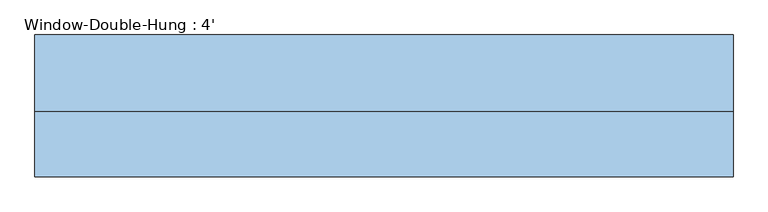
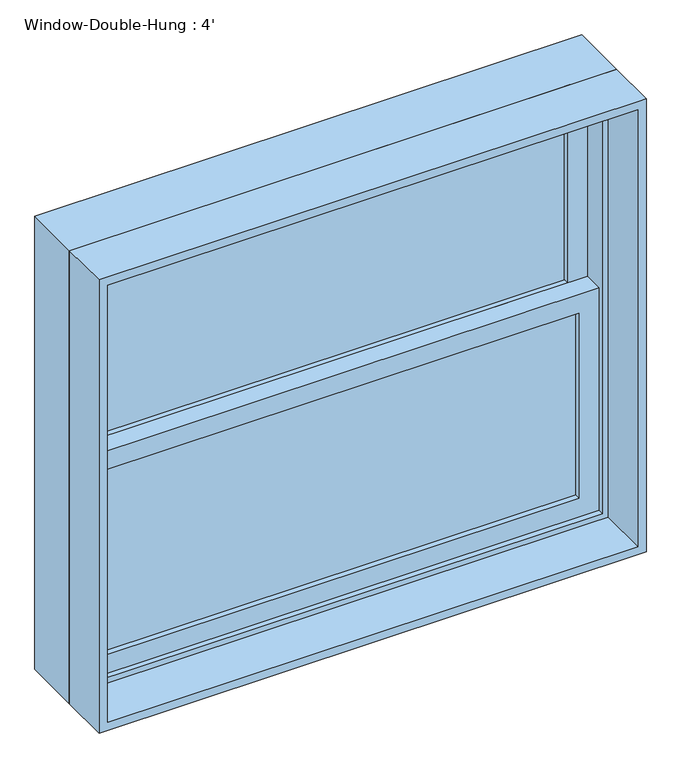
"""IFC4 building model written with IfcOpenShell, lengths in millimetres: window geometry, Window-Double-Hung : 4'."""

from ifc_helpers import new_model, si_unit, frame, origin, place, context, project, spatial, polyline, outline, extrude, source, transform, mapped, element, save


def window_double_hung_4_eadb0177(model_context):
    return source(origin(), model_context, "Body", "SweptSolid", [
        extrude(outline(polyline([(533.4, 44.45), (533.4, 38.1), (-533.4, 38.1), (-533.4, 44.45), (533.4, 44.45)])), frame((0.0, 0.0, 990.6), z_axis=(0.0, 0.0, 1.0), x_axis=(1.0, 0.0, 0.0)), (0.0, 0.0, 1.0), 434.975),
        extrude(outline(polyline([(-533.4, 31.75), (533.4, 31.75), (533.4, 25.4), (-533.4, 25.4), (-533.4, 31.75)])), frame((0.0, 0.0, 990.6), z_axis=(0.0, 0.0, 1.0), x_axis=(1.0, 0.0, 0.0)), (0.0, 0.0, 1.0), 434.975),
        extrude(outline(polyline([(533.4, 88.9), (533.4, 82.55), (-533.4, 82.55), (-533.4, 88.9), (533.4, 88.9)])), frame((0.0, 0.0, 1470.025), z_axis=(0.0, 0.0, 1.0), x_axis=(1.0, 0.0, 0.0)), (0.0, 0.0, 1.0), 434.975),
        extrude(outline(polyline([(-533.4, 76.2), (533.4, 76.2), (533.4, 69.85), (-533.4, 69.85), (-533.4, 76.2)])), frame((0.0, 0.0, 1470.025), z_axis=(0.0, 0.0, 1.0), x_axis=(1.0, 0.0, 0.0)), (0.0, 0.0, 1.0), 434.975),
        extrude(outline(polyline([(1470.025, -577.85), (946.15, -577.85), (946.15, 577.85), (1470.025, 577.85), (1470.025, -577.85)]), holes=[polyline([(1425.575, 533.4), (990.6, 533.4), (990.6, -533.4), (1425.575, -533.4), (1425.575, 533.4)])]), frame((0.0, 12.7, 0.0), z_axis=(0.0, 1.0, 0.0), x_axis=(0.0, 0.0, 1.0)), (0.0, 0.0, 1.0), 44.45),
        extrude(outline(polyline([(1949.45, -577.85), (1425.575, -577.85), (1425.575, 577.85), (1949.45, 577.85), (1949.45, -577.85)]), holes=[polyline([(1905.0, 533.4), (1470.025, 533.4), (1470.025, -533.4), (1905.0, -533.4), (1905.0, 533.4)])]), frame((0.0, 57.15, 0.0), z_axis=(0.0, 1.0, 0.0), x_axis=(0.0, 0.0, 1.0)), (0.0, 0.0, 1.0), 44.45),
        extrude(outline(polyline([(1981.2, -609.6), (914.4, -609.6), (914.4, 609.6), (1981.2, 609.6), (1981.2, -609.6)]), holes=[polyline([(1949.45, 577.85), (946.15, 577.85), (946.15, -577.85), (1949.45, -577.85), (1949.45, 577.85)])]), frame((0.0, 0.0, 0.0), z_axis=(0.0, 1.0, 0.0), x_axis=(0.0, 0.0, 1.0)), (0.0, 0.0, 1.0), 133.35),
        extrude(outline(polyline([(1981.2, 609.6), (1981.2, -609.6), (914.4, -609.6), (914.4, 609.6), (1981.2, 609.6)]), holes=[polyline([(1962.15, 590.55), (933.45, 590.55), (933.45, -590.55), (1962.15, -590.55), (1962.15, 590.55)])]), frame((0.0, -114.3, 0.0), z_axis=(0.0, 1.0, 0.0), x_axis=(0.0, 0.0, 1.0)), (0.0, 0.0, 1.0), 114.3),
    ])


if __name__ == "__main__":
    model = new_model("IFC4")
    model_context = context("Model", 3, world=origin())
    ifc_project = project(units=[si_unit("LENGTHUNIT", "METRE", prefix="MILLI")], contexts=[model_context])
    site = spatial("IfcSite", under=ifc_project)
    building = spatial("IfcBuilding", under=site)
    placement = place(None, origin())
    window_double_hung_4_shape = window_double_hung_4_eadb0177(model_context)
    element("IfcWindow", 1, ObjectType="Window-Double-Hung : 4'", at=placement, inside=building, context=model_context, shape_type="MappedRepresentation", body=[
        mapped(window_double_hung_4_shape, transform((0.0, 0.0, 0.0), x_axis=(1.0, 0.0, 0.0), y_axis=(0.0, 1.0, 0.0), z_axis=(0.0, 0.0, 1.0))),
    ])
    save(model, "model.ifc")

# Revit data of these elements
# Type "Window-Double-Hung : 4'"
#   Type Mark = "18"
#   Fire Rating = "0.5h"
#   Construction Type Id = "DG-DR"
#   Assembly Code = "B2020100"
#   Analytic Construction = "Double glazing - domestic"
#   Wall Thickness [instance default] = 0' - 6"
#   Window Inset [instance default] = 0' - 0"
#   Visual Light Transmittance = 0.81
#   Thermal Resistance (R) = 1.8146 (h·ft²·°F)/BTU
#   Solar Heat Gain Coefficient = 0.76
#   Muntin Width = 3' - 6"
#   Muntin Height = 1' - 5 1/8"
#   Interior Wall Closure [instance default] = 0' - 1 1/2"
#   Rough Width = 4' - 0 1/2"
#   Rough Height = 3' - 6 1/2"
#   Frame Extension [instance default] = 0' - 1 1/4"
#   Exterior Wall Closure [instance default] = 0' - 0 1/2"
#   Extension Jamb [instance default] = 0' - 1 1/2"
#   Heat Transfer Coefficient (U) = 0.5511 BTU/(h·ft²·°F)
#   Height = 3' - 6"
#   Width = 4' - 0"
#   Top Muntin Visibility = yes
#   Indicator Visibility [instance default] = yes
#   Extension Jamb Visibility [instance default] = yes
#   Interior Trim Visibility [instance default] = yes
#   Exterior Trim Visibility [instance default] = yes
#   Define Thermal Properties by = 1
#   Bottom Muntin Visibility = yes
#   Muntin Pattern = Muntin Pattern_2x2 : Muntin Pattern_2x2
#   Interior Trim Material = Wood - Stained
#   Interior Trim = Trim-Window-Interior-Flat : Picture Frame
#   Exterior Trim Material = Clad - White
#   Exterior Trim = Trim-Window-Exterior-Flat : with Sill
#   Glass Panel Material = Glass
#   Exterior Frame Material = Clad - White
#   Interior Frame Material = Wood - Stained
#   Wall Closure = (empty or 0)
# Element 1 (IfcWindow, "Window-Double-Hung : 4'")
#   Wall Thickness = 0' - 9"
#   Extension Jamb = 0' - 4 1/2"
#   Materials on its faces: "Wood - Stained", "Glass", "Clad - White"
# Materials
#   "Wood - Stained": class "Wood", colour RGB 224 178 126, transparency 0, Cost = 0
#   "Clad - White": class "Wood", colour RGB 242 242 238, transparency 0, Cost = 0
#   "Glass": class "Glass", colour RGB 0 128 192, transparency 0.75, Description = "Soda Lime Glass", Cost = 0
